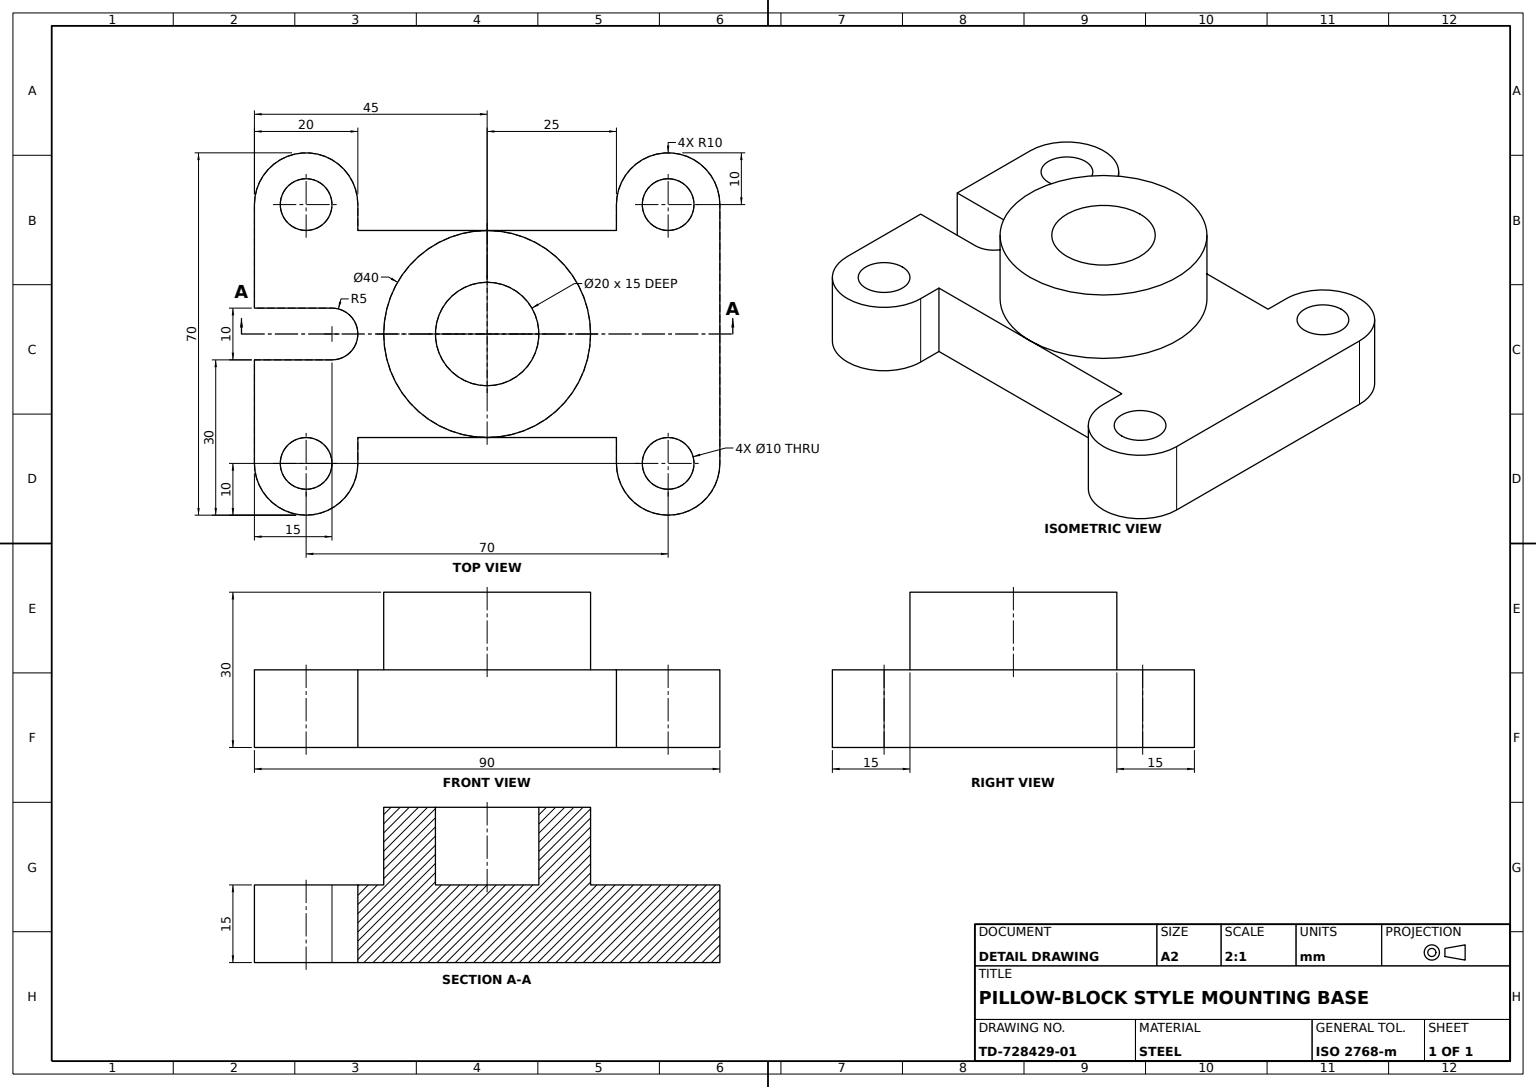
from build123d import *

# Parameters (mm, degrees)
BASE_PLATE_SKETCH_R         = 5
BASE_PLATE_DEPTH            = 15
PIVOT_BOSS_SKETCH_R         = 20
PIVOT_BOSS_SKETCH_R_2       = 10
PIVOT_BOSS_40_BORE_20_DEPTH = 15


with BuildPart() as part:
    # Base Plate Sketch → Base Plate (new body)
    with BuildSketch(Plane(origin=(0, 0, 0), x_dir=(1, 0, 0), z_dir=(0, 1, 0))):
        with BuildLine():
            Line((45, 25), (45, -25))
            ThreePointArc((45, -25), (35, -35), (25, -25))
            Line((25, -25), (25, -20))
            Line((25, -20), (-25, -20))
            Line((-25, -20), (-25, -25))
            ThreePointArc((-25, -25), (-35, -35), (-45, -25))
            Line((-45, -25), (-45, -5))
            Line((-45, -5), (-30, -5))
            ThreePointArc((-30, -5), (-25, 0), (-30, 5))
            Line((-30, 5), (-45, 5))
            Line((-45, 5), (-45, 25))
            ThreePointArc((-45, 25), (-35, 35), (-25, 25))
            Line((-25, 25), (-25, 20))
            Line((-25, 20), (25, 20))
            Line((25, 20), (25, 25))
            ThreePointArc((25, 25), (35, 35), (45, 25))
        make_face()
        with Locations(Location((35, -25, 0), (0, 0, 270))):
            Circle(BASE_PLATE_SKETCH_R, mode=Mode.SUBTRACT)
        with Locations(Location((-35, -25, 0), (0, 0, 270))):
            Circle(BASE_PLATE_SKETCH_R, mode=Mode.SUBTRACT)
        with Locations(Location((35, 25, 0), (0, 0, 270))):
            Circle(BASE_PLATE_SKETCH_R, mode=Mode.SUBTRACT)
        with Locations(Location((-35, 25, 0), (0, 0, 270))):
            Circle(BASE_PLATE_SKETCH_R, mode=Mode.SUBTRACT)
    extrude(amount=-BASE_PLATE_DEPTH)

    # Pivot Boss Sketch → Pivot Boss Ø40 Bore Ø20 (add)
    with BuildSketch(Plane(origin=(0, 0, 0), x_dir=(1, 0, 0), z_dir=(0, 1, 0))):
        with Locations(Location((0, 0, 0), (0, 0, 270))):
            Circle(PIVOT_BOSS_SKETCH_R)
        with Locations(Location((0, 0, 0), (0, 0, 270))):
            Circle(PIVOT_BOSS_SKETCH_R_2, mode=Mode.SUBTRACT)
    extrude(amount=PIVOT_BOSS_40_BORE_20_DEPTH)


solid = part.part
